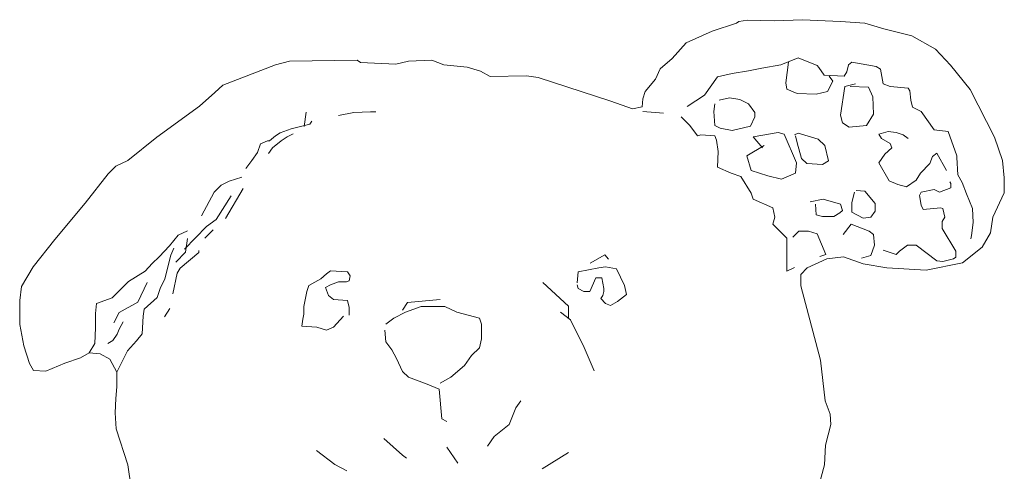
# Model space of a CAD drawing. Units: inches. Extents: x 638 to 1303, y 1 to 699.
# Tile 17 of 21: x 947.54 to 962.23, y 590.7 to 597.43. Entities that reach past the tile are written whole.
import ezdxf

# ---------------------------------------------------------------- set-up
doc = ezdxf.new("R2010")
doc.units = ezdxf.units.IN
doc.header["$MEASUREMENT"] = 0
doc.layers.add('A-FURN-ACCS', color=8, linetype='Continuous', lineweight=13)

msp = doc.modelspace()

# ---------------------------------------------------------------- linework, layer by layer
at = {"layer": 'A-FURN-ACCS'}
for p, q in [((958.23312, 597.38231), (957.87058, 597.26155)), ((958.26765, 597.40819), (958.23312, 597.38231)), ((958.39712, 597.42543), (958.26765, 597.40819)), ((958.79419, 597.41681), (958.39712, 597.42543)), ((959.21716, 597.43406), (958.79419, 597.41681)), ((959.78686, 597.40819), (959.21716, 597.43406)), ((960.1494, 597.38231), (959.78686, 597.40819)), ((960.43425, 597.29606), (960.1494, 597.38231)), ((957.87058, 597.26155), (957.48215, 597.08904)), ((960.84858, 597.19255), (960.43425, 597.29606)), ((961.20249, 596.99417), (960.84858, 597.19255)), ((957.48215, 597.08904), (957.27498, 596.85616)), ((961.42714, 596.75711), (961.20249, 596.99417)), ((951.35506, 596.76125), (950.56956, 596.45936)), ((951.56223, 596.813), (951.35506, 596.76125)), ((952.57216, 596.83025), (951.56223, 596.813)), ((952.62395, 596.79575), (952.57216, 596.83025)), ((953.1505, 596.76987), (952.62395, 596.79575)), ((953.3404, 596.813), (953.1505, 596.76987)), ((953.68567, 596.83025), (953.3404, 596.813)), ((953.86694, 596.76125), (953.68567, 596.83025)), ((954.21222, 596.72674), (953.86694, 596.76125)), ((957.27498, 596.85616), (957.09371, 596.7009)), ((958.60894, 596.71015), (958.89372, 596.76189)), ((958.89372, 596.76189), (959.15261, 596.86537)), ((959.01023, 596.80069), (958.97139, 596.49025)), ((959.15261, 596.86537), (959.4374, 596.74895)), ((959.4374, 596.74895), (959.46329, 596.72308)), ((959.87751, 596.65841), (959.90341, 596.76189)), ((959.90341, 596.76189), (959.95518, 596.80069)), ((959.95518, 596.80069), (960.31763, 596.73601)), ((960.31763, 596.73601), (960.38235, 596.69721)), ((961.72063, 596.39484), (961.42714, 596.75711)), ((954.41075, 596.66636), (954.21222, 596.72674)), ((954.55749, 596.58874), (954.41075, 596.66636)), ((955.1013, 596.59736), (954.55749, 596.58874)), ((955.27394, 596.57149), (955.1013, 596.59736)), ((957.09371, 596.7009), (957.02466, 596.54565)), ((957.94877, 596.5808), (958.16883, 596.63253)), ((958.16883, 596.63253), (958.41477, 596.67134)), ((958.41477, 596.67134), (958.60894, 596.71015)), ((959.46329, 596.72308), (959.54095, 596.60667)), ((959.54095, 596.60667), (959.83868, 596.59373)), ((959.6704, 596.51612), (959.61862, 596.59373)), ((959.83868, 596.59373), (959.87751, 596.65841)), ((960.38235, 596.69721), (960.42119, 596.47732)), ((950.56956, 596.45936), (950.44871, 596.34723)), ((956.36, 596.21788), (955.27394, 596.57149)), ((957.02466, 596.54565), (956.86928, 596.36451)), ((957.75459, 596.30916), (957.94877, 596.5808)), ((958.97139, 596.49025), (958.98433, 596.39971)), ((959.59273, 596.3609), (959.6704, 596.51612)), ((959.7869, 596.01166), (959.85163, 596.43851)), ((959.85163, 596.43851), (960.00696, 596.47732)), ((959.92929, 596.43851), (960.20113, 596.42558)), ((960.42119, 596.47732), (960.52474, 596.43851)), ((960.52474, 596.43851), (960.79658, 596.41264)), ((950.44871, 596.34723), (950.22032, 596.1456)), ((956.86928, 596.36451), (956.83476, 596.25238)), ((957.4957, 596.14101), (957.75459, 596.30916)), ((958.98433, 596.39971), (959.13967, 596.33503)), ((959.13967, 596.33503), (959.42445, 596.3221)), ((959.42445, 596.3221), (959.59273, 596.3609)), ((960.20113, 596.42558), (960.26585, 596.28329)), ((960.79658, 596.41264), (960.82247, 596.37384)), ((960.82247, 596.37384), (960.83542, 596.23155)), ((962.08316, 595.67893), (961.72063, 596.39484)), ((950.22032, 596.1456), (949.58156, 595.67983)), ((956.67939, 596.10575), (956.36, 596.21788)), ((956.83476, 596.25238), (956.82612, 596.13163)), ((957.89699, 596.0634), (957.90993, 596.17981)), ((957.97465, 596.23155), (958.12999, 596.27036)), ((958.12999, 596.27036), (958.28533, 596.24449)), ((958.28533, 596.24449), (958.41477, 596.17981)), ((958.41477, 596.17981), (958.50539, 596.05047)), ((960.26585, 596.28329), (960.2788, 596.02459)), ((960.83542, 596.23155), (960.8613, 596.12807)), ((951.81136, 596.05425), (951.78051, 595.83848)), ((952.29286, 596.00644), (952.52429, 596.04725)), ((952.52429, 596.04725), (952.76933, 596.06085)), ((952.76933, 596.06085), (952.85101, 596.06085)), ((956.82612, 596.13163), (956.67939, 596.10575)), ((956.83553, 596.0634), (957.1462, 596.03753)), ((957.90993, 595.85644), (957.89699, 596.0634)), ((958.50539, 596.05047), (958.50539, 595.98579)), ((959.81279, 595.89525), (959.7869, 596.01166)), ((960.2788, 596.02459), (960.17524, 595.85644)), ((960.8613, 596.12807), (960.99075, 596.0634)), ((960.99075, 596.0634), (961.18492, 595.79177)), ((951.5868, 595.80344), (951.86636, 595.87695)), ((951.86636, 595.87695), (951.89579, 595.92106)), ((957.40509, 595.98579), (957.53454, 595.85644)), ((957.53454, 595.85644), (957.65104, 595.70122)), ((957.9876, 595.81764), (957.90993, 595.85644)), ((958.50539, 595.98579), (958.44066, 595.8435)), ((959.91635, 595.83057), (959.81279, 595.89525)), ((960.17524, 595.85644), (959.91635, 595.83057)), ((951.35138, 595.70052), (951.42495, 595.74463)), ((951.42495, 595.74463), (951.5868, 595.80344)), ((951.61622, 595.72993), (951.52794, 595.68582)), ((957.65104, 595.70122), (957.70282, 595.71416)), ((957.70282, 595.71416), (957.90993, 595.70122)), ((958.16883, 595.77883), (957.9876, 595.81764)), ((958.44066, 595.8435), (958.16883, 595.77883)), ((958.85489, 595.75296), (958.47949, 595.68829)), ((958.9455, 595.72709), (958.85489, 595.75296)), ((959.12673, 595.30024), (958.9455, 595.72709)), ((959.10084, 595.71416), (959.15261, 595.74003)), ((959.15261, 595.74003), (959.45034, 595.64948)), ((960.49885, 595.7659), (960.35647, 595.72709)), ((960.35647, 595.72709), (960.3953, 595.66242)), ((960.61536, 595.75296), (960.49885, 595.7659)), ((960.71891, 595.71416), (960.61536, 595.75296)), ((960.79658, 595.66242), (960.71891, 595.71416)), ((961.18492, 595.79177), (961.39203, 595.7659)), ((961.39203, 595.7659), (961.52148, 595.40372)), ((949.58156, 595.67983), (949.14997, 595.33481)), ((951.08653, 595.45058), (951.13067, 595.5829)), ((951.13067, 595.5829), (951.23367, 595.62701)), ((951.23367, 595.62701), (951.26309, 595.62701)), ((951.26309, 595.62701), (951.35138, 595.70052)), ((951.43966, 595.62701), (951.30724, 595.52409)), ((951.52794, 595.68582), (951.43966, 595.62701)), ((957.90993, 595.70122), (957.93582, 595.63655)), ((957.93582, 595.63655), (957.96171, 595.46839)), ((958.64777, 595.55894), (958.38888, 595.40372)), ((958.47949, 595.68829), (958.62189, 595.52013)), ((959.13967, 595.59774), (959.11378, 595.70122)), ((959.20439, 595.36492), (959.13967, 595.59774)), ((959.45034, 595.64948), (959.5539, 595.55894)), ((959.5539, 595.55894), (959.60568, 595.32611)), ((960.3953, 595.66242), (960.52474, 595.58481)), ((960.52474, 595.58481), (960.55063, 595.52013)), ((962.20401, 595.33391), (962.08316, 595.67893)), ((950.99825, 595.33295), (951.08653, 595.45058)), ((951.30724, 595.52409), (951.24838, 595.43587)), ((957.96171, 595.46839), (957.94877, 595.23556)), ((960.44708, 595.42959), (960.35647, 595.30024)), ((960.55063, 595.52013), (960.44708, 595.42959)), ((961.15903, 595.39078), (961.22375, 595.44253)), ((961.22375, 595.44253), (961.36614, 595.18383)), ((949.14997, 595.33481), (948.9687, 595.24856)), ((950.90997, 595.21533), (950.99825, 595.33295)), ((958.38888, 595.40372), (958.45361, 595.18383)), ((959.11378, 595.14502), (959.12673, 595.30024)), ((959.28206, 595.2873), (959.20439, 595.36492)), ((959.51507, 595.27437), (959.28206, 595.2873)), ((959.60568, 595.32611), (959.51507, 595.27437)), ((960.35647, 595.30024), (960.5118, 595.02861)), ((960.9778, 595.14502), (961.1202, 595.2873)), ((961.1202, 595.2873), (961.15903, 595.39078)), ((961.52148, 595.40372), (961.52148, 595.37785)), ((961.52148, 595.37785), (961.53442, 595.11915)), ((962.22991, 595.07515), (962.20401, 595.33391)), ((948.85649, 595.13643), (948.51121, 594.69653)), ((948.9687, 595.24856), (948.85649, 595.13643)), ((957.94877, 595.23556), (958.15588, 595.14502)), ((958.15588, 595.14502), (958.29827, 595.09328)), ((958.45361, 595.18383), (958.69955, 595.10622)), ((958.90667, 595.05448), (959.11378, 595.14502)), ((960.91308, 595.04154), (960.9778, 595.14502)), ((961.53442, 595.11915), (961.59914, 595.00274)), ((950.54212, 594.96539), (950.65984, 595.0242)), ((950.65984, 595.0242), (950.85111, 595.08301)), ((958.29827, 595.09328), (958.45361, 594.84752)), ((958.69955, 595.10622), (958.90667, 595.05448)), ((960.5118, 595.02861), (960.64125, 594.97687)), ((960.64125, 594.97687), (960.77069, 594.93806)), ((960.77069, 594.93806), (960.91308, 595.04154)), ((961.41792, 595.01567), (961.43086, 594.9898)), ((961.43086, 594.9898), (961.43086, 594.92513)), ((961.59914, 595.00274), (961.66387, 594.83458)), ((962.22991, 594.85089), (962.22991, 595.07515)), ((950.24785, 594.5096), (950.43913, 594.86247)), ((950.43913, 594.86247), (950.54212, 594.96539)), ((950.87051, 594.91376), (950.60831, 594.4668)), ((958.45361, 594.84752), (958.47949, 594.75697)), ((959.95518, 594.70523), (959.99401, 594.86045)), ((960.01991, 594.88632), (960.14935, 594.87339)), ((960.14935, 594.87339), (960.30469, 594.6923)), ((960.99075, 594.86045), (960.96486, 594.80871)), ((961.18492, 594.89926), (960.99075, 594.86045)), ((961.26258, 594.86045), (961.18492, 594.89926)), ((961.43086, 594.92513), (961.26258, 594.86045)), ((961.66387, 594.83458), (961.75448, 594.61469)), ((962.05727, 594.48863), (962.22991, 594.85089)), ((948.51121, 594.69653), (948.06235, 594.15313)), ((950.68926, 594.80366), (950.46856, 594.45079)), ((958.47949, 594.75697), (958.77722, 594.62762)), ((959.33384, 594.71817), (959.52801, 594.75697)), ((959.42445, 594.52414), (959.41151, 594.67936)), ((959.52801, 594.75697), (959.7869, 594.67936)), ((959.7869, 594.67936), (959.81279, 594.58882)), ((959.95518, 594.56295), (959.95518, 594.70523)), ((960.30469, 594.6923), (960.30469, 594.57588)), ((960.96486, 594.80871), (960.99075, 594.66643)), ((958.77722, 594.62762), (958.80311, 594.48534)), ((959.77396, 594.55002), (959.68335, 594.49827)), ((959.81279, 594.58882), (959.77396, 594.55002)), ((960.12346, 594.47241), (959.95518, 594.56295)), ((960.30469, 594.57588), (960.23996, 594.48534)), ((960.99075, 594.66643), (961.01664, 594.60175)), ((961.01664, 594.60175), (961.27553, 594.62762)), ((961.27553, 594.62762), (961.31436, 594.61469)), ((961.31436, 594.61469), (961.34026, 594.48534)), ((961.75448, 594.61469), (961.76743, 594.40773)), ((950.46856, 594.45079), (950.32142, 594.34788)), ((958.80311, 594.48534), (958.77722, 594.38186)), ((958.77722, 594.38186), (958.98433, 594.1749)), ((959.51507, 594.49827), (959.42445, 594.52414)), ((959.68335, 594.49827), (959.51507, 594.49827)), ((959.82573, 594.22664), (959.94224, 594.38186)), ((959.94224, 594.38186), (960.21407, 594.27838)), ((960.23996, 594.48534), (960.12346, 594.47241)), ((961.34026, 594.48534), (961.30142, 594.42066)), ((961.30142, 594.42066), (961.30142, 594.31718)), ((961.76743, 594.40773), (961.74154, 594.21371)), ((962.02274, 594.25574), (962.05727, 594.48863)), ((949.90087, 594.21695), (950.03897, 594.28595)), ((950.32142, 594.34788), (949.99772, 594.00971)), ((950.42323, 594.29727), (950.29984, 594.17397)), ((959.07495, 594.18784), (959.16556, 594.27838)), ((959.16556, 594.27838), (959.30795, 594.27838)), ((959.30795, 594.27838), (959.4374, 594.23958)), ((959.4374, 594.23958), (959.56684, 593.92914)), ((960.21407, 594.27838), (960.2788, 594.22664)), ((961.30142, 594.31718), (961.50854, 593.98088)), ((961.9019, 594.04011), (962.02274, 594.25574)), ((948.06235, 594.15313), (947.73434, 593.74774)), ((949.77139, 594.06169), (949.90087, 594.21695)), ((950.01243, 593.96561), (950.04186, 594.17144)), ((958.98433, 594.1749), (958.98433, 594.00675)), ((960.2788, 594.22664), (960.29174, 594.07142)), ((961.74154, 594.21371), (961.72859, 594.16197)), ((949.61601, 593.89781), (949.77139, 594.06169)), ((949.79172, 593.9215), (949.83587, 594.02442)), ((949.8653, 593.81858), (950.01243, 593.96561)), ((950.20729, 593.9582), (949.92967, 593.72702)), ((950.20729, 593.98903), (950.20729, 593.9582)), ((958.98433, 594.00675), (958.98433, 593.68337)), ((960.29174, 594.07142), (960.23996, 593.9162)), ((960.61536, 593.92914), (960.42119, 593.99381)), ((960.66714, 593.98088), (960.61536, 593.92914)), ((960.78364, 594.07142), (960.66714, 593.98088)), ((960.91308, 594.07142), (960.78364, 594.07142)), ((961.22375, 593.8386), (960.91308, 594.07142)), ((961.50854, 593.98088), (961.50854, 593.89033)), ((961.60841, 593.80722), (961.9019, 594.04011)), ((949.40885, 593.68217), (949.51243, 593.7943)), ((949.51243, 593.7943), (949.61601, 593.89781)), ((949.70344, 593.56864), (949.79172, 593.9215)), ((956.04764, 593.79919), (956.26966, 593.92343)), ((956.26966, 593.92343), (956.32295, 593.86131)), ((959.28644, 593.72959), (959.57992, 593.8676)), ((959.56684, 593.92914), (959.47623, 593.90327)), ((959.57992, 593.8676), (959.83025, 593.89347)), ((959.83025, 593.89347), (960.12373, 593.78997)), ((960.23996, 593.9162), (960.09757, 593.8774)), ((961.0646, 593.69509), (961.60841, 593.80722)), ((961.31436, 593.82566), (961.22375, 593.8386)), ((961.4697, 593.86446), (961.31436, 593.82566)), ((961.50854, 593.89033), (961.4697, 593.86446)), ((947.73434, 593.74774), (947.5617, 593.45447)), ((949.15852, 593.52691), (949.40885, 593.68217)), ((949.8834, 593.64996), (949.8217, 593.34172)), ((949.92967, 593.72702), (949.8834, 593.64996)), ((952.11649, 593.64215), (952.17535, 593.68626)), ((952.17535, 593.68626), (952.42548, 593.67155)), ((952.42548, 593.67155), (952.46962, 593.61274)), ((955.85377, 593.50982), (955.86848, 593.67155)), ((955.86848, 593.67155), (956.17747, 593.73036)), ((956.17747, 593.73036), (956.28046, 593.74507)), ((956.28046, 593.74507), (956.44232, 593.71566)), ((956.44232, 593.71566), (956.56002, 593.46572)), ((958.98433, 593.68337), (959.10084, 593.73512)), ((959.19149, 593.63471), (959.28644, 593.72959)), ((960.12373, 593.78997), (960.47764, 593.72959)), ((960.47764, 593.72959), (961.0646, 593.69509)), ((949.01178, 593.38028), (949.15852, 593.52691)), ((949.43611, 593.51125), (949.2973, 593.21842)), ((949.62988, 593.42161), (949.70344, 593.56864)), ((951.85164, 593.46572), (952.0282, 593.56864)), ((952.0282, 593.56864), (952.11649, 593.64215)), ((952.29305, 593.52452), (952.17535, 593.48042)), ((952.41077, 593.52452), (952.29305, 593.52452)), ((952.4549, 593.53923), (952.41077, 593.52452)), ((952.46962, 593.61274), (952.4549, 593.53923)), ((955.3454, 593.51092), (955.72605, 593.15982)), ((956.13333, 593.58334), (956.04504, 593.3775)), ((956.22161, 593.58334), (956.13333, 593.58334)), ((956.25103, 593.42161), (956.22161, 593.58334)), ((959.19217, 593.46471), (959.19149, 593.63471)), ((947.5617, 593.45447), (947.53573, 593.24227)), ((948.91683, 593.2854), (949.01178, 593.38028)), ((949.58574, 593.28929), (949.62988, 593.42161)), ((951.77807, 593.15696), (951.82221, 593.3775)), ((951.82221, 593.3775), (951.85164, 593.46572)), ((952.17535, 593.48042), (952.10178, 593.43631)), ((952.10178, 593.43631), (952.14592, 593.31869)), ((955.86848, 593.42161), (955.85377, 593.48042)), ((955.95676, 593.3775), (955.86848, 593.42161)), ((956.04504, 593.3775), (955.95676, 593.3775)), ((956.23632, 593.31869), (956.25103, 593.3775)), ((956.25103, 593.3775), (956.25103, 593.42161)), ((956.56002, 593.46572), (956.58945, 593.33339)), ((959.48565, 592.35204), (959.19217, 593.46471)), ((947.53573, 593.24227), (947.53573, 592.88864)), ((948.68377, 593.19915), (948.91683, 593.2854)), ((949.2973, 593.21842), (949.01967, 593.0643)), ((949.39446, 593.11285), (949.58574, 593.28929)), ((952.14592, 593.31869), (952.21948, 593.25988)), ((952.21948, 593.25988), (952.42548, 593.24517)), ((952.42548, 593.24517), (952.4549, 593.14226)), ((953.24944, 593.09815), (953.32301, 593.21577)), ((953.32301, 593.21577), (953.80856, 593.25988)), ((956.2069, 593.27458), (956.23632, 593.31869)), ((956.28046, 593.20107), (956.2069, 593.27458)), ((956.45703, 593.23047), (956.35403, 593.17166)), ((956.58945, 593.33339), (956.45703, 593.23047)), ((948.66651, 593.05252), (948.68377, 593.19915)), ((949.01967, 593.0643), (948.94255, 592.91018)), ((949.37975, 593.00993), (949.39446, 593.11285)), ((949.77543, 593.12595), (949.69832, 593.00265)), ((951.77807, 593.03934), (951.77807, 593.15696)), ((952.4549, 593.14226), (952.4549, 593.02463)), ((953.11702, 592.98053), (953.29358, 593.06874)), ((953.29358, 593.06874), (953.529, 593.15696)), ((953.529, 593.15696), (953.632, 593.15696)), ((953.632, 593.15696), (953.88213, 593.15696)), ((953.88213, 593.15696), (954.05869, 593.06874)), ((954.05869, 593.06874), (954.39711, 592.98053)), ((955.60893, 593.07205), (955.75533, 592.95502)), ((955.72605, 593.15982), (955.72605, 592.98427)), ((956.35403, 593.17166), (956.28046, 593.20107)), ((948.66651, 592.83688), (948.66651, 593.05252)), ((949.08136, 592.92559), (949.01967, 592.8177)), ((949.36503, 592.74528), (949.37975, 593.00993)), ((951.74864, 592.86291), (951.76336, 592.96582)), ((951.76336, 592.96582), (951.77807, 593.03934)), ((952.36662, 593.00993), (952.21948, 592.8482)), ((952.99931, 592.89231), (953.11702, 592.98053)), ((954.39711, 592.98053), (954.42654, 592.89231)), ((955.75533, 592.95502), (955.96029, 592.5454)), ((947.53573, 592.88864), (947.59615, 592.56949)), ((948.65788, 592.60399), (948.66651, 592.83688)), ((949.01967, 592.8177), (948.98882, 592.74065)), ((951.96935, 592.8482), (951.74864, 592.86291)), ((952.11649, 592.8041), (951.96935, 592.8482)), ((952.21948, 592.8482), (952.11649, 592.8041)), ((952.9846, 592.8041), (952.99931, 592.62766)), ((954.42654, 592.89231), (954.42654, 592.67177)), ((948.92713, 592.64817), (948.85001, 592.60194)), ((948.98882, 592.74065), (948.92713, 592.64817)), ((949.14433, 592.49534), (949.27675, 592.64236)), ((949.27675, 592.64236), (949.36503, 592.74528)), ((952.99931, 592.62766), (953.08759, 592.51004)), ((954.42654, 592.67177), (954.39711, 592.53945)), ((947.59615, 592.56949), (947.68247, 592.30211)), ((948.57155, 592.46599), (948.65788, 592.60399)), ((948.98588, 592.17273), (949.14433, 592.49534)), ((953.08759, 592.51004), (953.16116, 592.37772)), ((954.39711, 592.53945), (954.2794, 592.42183)), ((955.96029, 592.5454), (956.10669, 592.1943)), ((948.20902, 592.31073), (948.44208, 592.38836)), ((948.44208, 592.38836), (948.57155, 592.46599)), ((948.57155, 592.46599), (948.73556, 592.44874)), ((948.73556, 592.44874), (948.8823, 592.37111)), ((948.8823, 592.37111), (948.98588, 592.17273)), ((953.16116, 592.37772), (953.24944, 592.18658)), ((954.2794, 592.42183), (954.17641, 592.2748)), ((959.55471, 591.74826), (959.48565, 592.35204)), ((947.68247, 592.30211), (947.7429, 592.1986)), ((947.7429, 592.1986), (947.92416, 592.18998)), ((947.92416, 592.18998), (948.20902, 592.31073)), ((953.24944, 592.18658), (953.33772, 592.09837)), ((954.17641, 592.2748), (953.97041, 592.09837)), ((948.98588, 592.17273), (948.98588, 591.95709)), ((953.33772, 592.09837), (953.61729, 591.99545)), ((953.97041, 592.09837), (953.80856, 592.01015)), ((948.98588, 591.95709), (948.96862, 591.78458)), ((953.61729, 591.99545), (953.79385, 591.92194)), ((953.79385, 591.92194), (953.83799, 591.48086)), ((948.96862, 591.78458), (948.95999, 591.56894)), ((955.01508, 591.7455), (954.94152, 591.64259)), ((959.6324, 591.54987), (959.55471, 591.74826)), ((954.94152, 591.64259), (954.83852, 591.39264)), ((948.95999, 591.56894), (948.97725, 591.32744)), ((953.83799, 591.48086), (953.91156, 591.43675)), ((959.64103, 591.39462), (959.6324, 591.54987)), ((948.97725, 591.32744), (949.14989, 590.79266)), ((954.83852, 591.39264), (954.61782, 591.21621)), ((959.56334, 591.0841), (959.64103, 591.39462)), ((952.96988, 591.1868), (953.24944, 590.93686)), ((954.61782, 591.21621), (954.51482, 591.06918)), ((951.96615, 591.00532), (952.23677, 590.79499)), ((953.91156, 591.05448), (954.07341, 590.81924)), ((959.54608, 590.79084), (959.56334, 591.0841)), ((953.24944, 590.93686), (953.3083, 590.89275)), ((955.72477, 590.97527), (955.33388, 590.7349)), ((949.14989, 590.79266), (949.20169, 590.44764)), ((952.23677, 590.79499), (952.41718, 590.70485)), ((959.42362, 590.34166), (959.54608, 590.79084))]:
    msp.add_line(p, q, dxfattribs=at)

doc.saveas('drawing.dxf')
